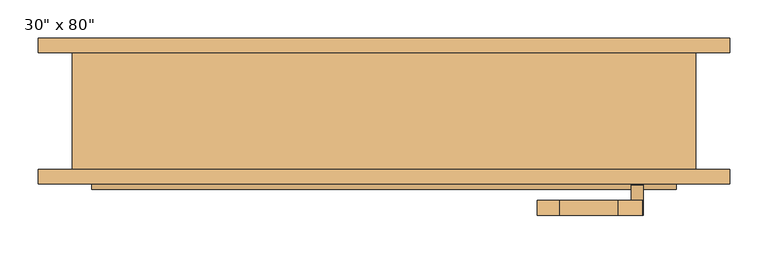
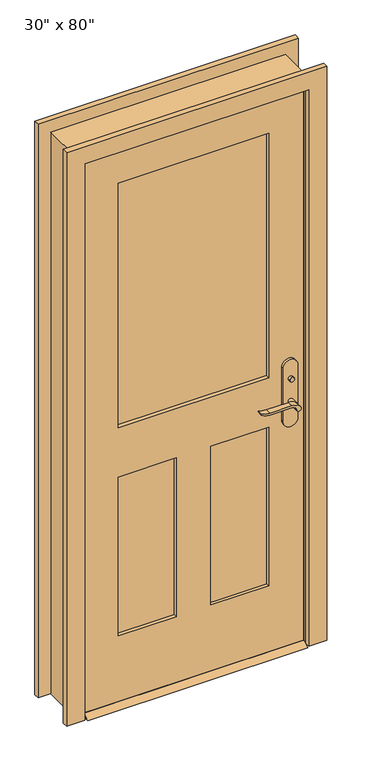
"""IFC4 building model written with IfcOpenShell, lengths in millimetres: door geometry."""

from ifc_helpers import new_model, si_unit, point, frame, frame_2d, origin, place, context, project, spatial, polyline, circle_curve, trimmed, segment, composite_curve, outline, extrude, faceted_brep, source, transform, mapped, element, save


def door_ce1fc124(model_context):
    return source(origin(), model_context, "Body", "SolidModel", [
        extrude(outline(polyline([(-38.1, 12.7), (-12.7, 0.0), (-98.425, 0.0), (-73.025, 12.7), (-38.1, 12.7)])), frame((-381.0, 0.0, 0.0), z_axis=(1.0, 0.0, 0.0), x_axis=(0.0, 1.0, 0.0)), (0.0, 0.0, 1.0), 762.0),
        extrude(outline(polyline([(335.2, -18.1), (335.2, -28.1), (325.2, -28.1), (325.2, -18.1), (335.2, -18.1)])), frame((0.0, 0.0, 981.9), z_axis=(0.0, 0.0, 1.0), x_axis=(1.0, 0.0, 0.0)), (0.0, 0.0, 1.0), 30.0),
        extrude(outline(composite_curve([segment(trimmed(circle_curve(frame_2d((996.9, 330.2)), 8.0), [point((996.9, 322.2))], [point((996.9, 338.2))], False, "CARTESIAN"), True, "CONTINUOUS"), segment(trimmed(circle_curve(frame_2d((996.9, 330.2)), 8.0), [point((996.9, 338.2))], [point((996.9, 322.2))], False, "CARTESIAN"), True, "CONTINUOUS")], self_intersect=False)), frame((0.0, -93.025, 0.0), z_axis=(0.0, 1.0, 0.0), x_axis=(0.0, 0.0, 1.0)), (0.0, 0.0, 1.0), 10.0),
        extrude(outline(composite_curve([segment(trimmed(circle_curve(frame_2d((897.1555521, 306.5324871)), 37.2832219), [point((919.0523287, 336.7081363))], [point((934.4, 304.8325667))], False, "CARTESIAN"), True, "CONTINUOUS"), segment(polyline([(934.4, 304.8325667), (934.4, 228.5564091)]), True, "CONTINUOUS"), segment(trimmed(circle_curve(frame_2d((1017.6850638, 228.6227909)), 83.2850902), [point((934.4, 228.5564091))], [point((939.4, 200.2))], True, "CARTESIAN"), True, "CONTINUOUS"), segment(polyline([(939.4, 200.2), (936.6135558, 200.2)]), True, "CONTINUOUS"), segment(trimmed(circle_curve(frame_2d((986.6709207, 232.1396612)), 59.3791355), [point((936.6135558, 200.2))], [point((927.4, 228.5564091))], False, "CARTESIAN"), True, "CONTINUOUS"), segment(polyline([(927.4, 228.5564091), (927.4, 304.8138099)]), True, "CONTINUOUS"), segment(trimmed(circle_curve(frame_2d((909.2738613, 304.8138099)), 18.1261387), [point((927.4, 304.8138099))], [point((914.4, 322.2))], True, "CARTESIAN"), True, "CONTINUOUS"), segment(trimmed(circle_curve(frame_2d((914.4, 330.2)), 8.0), [point((914.4, 322.2))], [point((919.0523287, 336.7081363))], False, "CARTESIAN"), True, "CONTINUOUS")], self_intersect=False)), frame((0.0, 1.9, 0.0), z_axis=(0.0, 1.0, 0.0), x_axis=(0.0, 0.0, 1.0)), (0.0, 0.0, 1.0), 20.0),
        extrude(outline(composite_curve([segment(trimmed(circle_curve(frame_2d((914.4, 330.2)), 8.0), [point((914.3999903, 322.2))], [point((919.0523287, 336.7081363))], False, "CARTESIAN"), True, "CONTINUOUS"), segment(trimmed(circle_curve(frame_2d((897.1555521, 306.5324871)), 37.2832219), [point((919.0523287, 336.7081363))], [point((934.4, 304.8325667))], False, "CARTESIAN"), True, "CONTINUOUS"), segment(polyline([(934.4, 304.8325667), (934.4, 228.5564091)]), True, "CONTINUOUS"), segment(trimmed(circle_curve(frame_2d((1017.6850638, 228.6227909)), 83.2850902), [point((934.4, 228.5564091))], [point((939.4, 200.2))], True, "CARTESIAN"), True, "CONTINUOUS"), segment(polyline([(939.4, 200.2), (936.6135558, 200.2)]), True, "CONTINUOUS"), segment(trimmed(circle_curve(frame_2d((986.6709207, 232.1396612)), 59.3791355), [point((936.6135558, 200.2))], [point((927.4, 228.5564091))], False, "CARTESIAN"), True, "CONTINUOUS"), segment(polyline([(927.4, 228.5564091), (927.4, 304.8138122)]), True, "CONTINUOUS"), segment(trimmed(circle_curve(frame_2d((909.2738682, 304.8138122)), 18.1261318), [point((927.4, 304.8138122))], [point((914.3999903, 322.2))], True, "CARTESIAN"), True, "CONTINUOUS")], self_intersect=False)), frame((0.0, -133.025, 0.0), z_axis=(0.0, 1.0, 0.0), x_axis=(0.0, 0.0, 1.0)), (0.0, 0.0, 1.0), 20.0),
        extrude(outline(composite_curve([segment(trimmed(circle_curve(frame_2d((914.4, 330.2)), 8.0), [point((914.4, 322.2))], [point((914.4, 338.2))], False, "CARTESIAN"), True, "CONTINUOUS"), segment(trimmed(circle_curve(frame_2d((914.4, 330.2)), 8.0), [point((914.4, 338.2))], [point((914.4, 322.2))], False, "CARTESIAN"), True, "CONTINUOUS")], self_intersect=False)), frame((0.0, -28.1, 0.0), z_axis=(0.0, 1.0, 0.0), x_axis=(0.0, 0.0, 1.0)), (0.0, 0.0, 1.0), 30.0),
        extrude(outline(composite_curve([segment(trimmed(circle_curve(frame_2d((914.4, 330.2)), 8.0), [point((914.4, 322.2))], [point((914.4, 338.2))], False, "CARTESIAN"), True, "CONTINUOUS"), segment(trimmed(circle_curve(frame_2d((914.4, 330.2)), 8.0), [point((914.4, 338.2))], [point((914.4, 322.2))], False, "CARTESIAN"), True, "CONTINUOUS")], self_intersect=False)), frame((0.0, -113.025, 0.0), z_axis=(0.0, 1.0, 0.0), x_axis=(0.0, 0.0, 1.0)), (0.0, 0.0, 1.0), 30.0),
        extrude(outline(composite_curve([segment(polyline([(844.4, 355.2), (1039.4, 355.2)]), True, "CONTINUOUS"), segment(trimmed(circle_curve(frame_2d((1039.4, 330.2)), 25.0), [point((1039.4, 355.2))], [point((1039.4, 305.2))], False, "CARTESIAN"), True, "CONTINUOUS"), segment(polyline([(1039.4, 305.2), (844.4, 305.2)]), True, "CONTINUOUS"), segment(trimmed(circle_curve(frame_2d((844.4, 330.2)), 25.0), [point((844.4, 305.2))], [point((844.4, 355.2))], False, "CARTESIAN"), True, "CONTINUOUS")], self_intersect=False)), frame((0.0, -38.1, 0.0), z_axis=(0.0, 1.0, 0.0), x_axis=(0.0, 0.0, 1.0)), (0.0, 0.0, 1.0), 10.0),
        extrude(outline(composite_curve([segment(polyline([(844.4, 355.2), (1039.4, 355.2)]), True, "CONTINUOUS"), segment(trimmed(circle_curve(frame_2d((1039.4, 330.2)), 25.0), [point((1039.4, 355.2))], [point((1039.4, 305.2))], False, "CARTESIAN"), True, "CONTINUOUS"), segment(polyline([(1039.4, 305.2), (844.4, 305.2)]), True, "CONTINUOUS"), segment(trimmed(circle_curve(frame_2d((844.4, 330.2)), 25.0), [point((844.4, 305.2))], [point((844.4, 355.2))], False, "CARTESIAN"), True, "CONTINUOUS")], self_intersect=False)), frame((0.0, -83.025, 0.0), z_axis=(0.0, 1.0, 0.0), x_axis=(0.0, 0.0, 1.0)), (0.0, 0.0, 1.0), 10.0),
        extrude(outline(polyline([(2032.0, -381.0), (12.7, -381.0), (12.7, 381.0), (2032.0, 381.0), (2032.0, -381.0)]), holes=[polyline([(1016.0, -260.35), (1911.35, -260.35), (1911.35, 260.35), (1016.0, 260.35), (1016.0, -260.35)]), polyline([(835.025, -60.325), (254.0, -60.325), (254.0, -260.35), (835.025, -260.35), (835.025, -60.325)]), polyline([(835.025, 260.35), (254.0, 260.35), (254.0, 60.325), (835.025, 60.325), (835.025, 260.35)])]), frame((0.0, -73.025, 0.0), z_axis=(0.0, 1.0, 0.0), x_axis=(0.0, 0.0, 1.0)), (0.0, 0.0, 1.0), 34.925),
        faceted_brep([(406.4, -73.025, 0.0), (381.0, -73.025, 0.0), (381.0, -38.1, 0.0), (368.3, -38.1, 0.0), (368.3, -3.175, 0.0), (381.0, -3.175, 0.0), (381.0, 79.375, 0.0), (406.4, 79.375, 0.0), (406.4, 79.375, 2057.4), (406.4, -73.025, 2057.4), (381.0, 79.375, 2032.0), (-381.0, 79.375, 2032.0), (-381.0, 79.375, 0.0), (-406.4, 79.375, 0.0), (-406.4, 79.375, 2057.4), (381.0, -3.175, 2032.0), (368.3, -3.175, 2019.3), (-368.3, -3.175, 2019.3), (-368.3, -3.175, 0.0), (-381.0, -3.175, 0.0), (-381.0, -3.175, 2032.0), (368.3, -38.1, 2019.3), (381.0, -38.1, 2032.0), (-381.0, -38.1, 2032.0), (-381.0, -38.1, 0.0), (-368.3, -38.1, 0.0), (-368.3, -38.1, 2019.3), (381.0, -73.025, 2032.0), (-406.4, -73.025, 2057.4), (-406.4, -73.025, 0.0), (-381.0, -73.025, 0.0), (-381.0, -73.025, 2032.0)], [[[0, 1, 2, 3, 4, 5, 6, 7]], [[7, 8, 9, 0]], [[6, 10, 11, 12, 13, 14, 8, 7]], [[5, 15, 10, 6]], [[4, 16, 17, 18, 19, 20, 15, 5]], [[3, 21, 16, 4]], [[2, 22, 23, 24, 25, 26, 21, 3]], [[1, 27, 22, 2]], [[0, 9, 28, 29, 30, 31, 27, 1]], [[8, 14, 28, 9]], [[15, 20, 11, 10]], [[21, 26, 17, 16]], [[27, 31, 23, 22]], [[29, 13, 12, 19, 18, 25, 24, 30]], [[14, 13, 29, 28]], [[20, 19, 12, 11]], [[26, 25, 18, 17]], [[31, 30, 24, 23]]]),
        extrude(outline(polyline([(-60.325, -49.7416667), (-60.325, -61.3833333), (-260.35, -61.3833333), (-260.35, -49.7416667), (-60.325, -49.7416667)])), frame((0.0, 0.0, 254.0), z_axis=(0.0, 0.0, 1.0), x_axis=(1.0, 0.0, 0.0)), (0.0, 0.0, 1.0), 581.025),
        extrude(outline(polyline([(260.35, -49.7416667), (260.35, -61.3833333), (60.325, -61.3833333), (60.325, -49.7416667), (260.35, -49.7416667)])), frame((0.0, 0.0, 254.0), z_axis=(0.0, 0.0, 1.0), x_axis=(1.0, 0.0, 0.0)), (0.0, 0.0, 1.0), 581.025),
        extrude(outline(polyline([(260.35, -52.07), (260.35, -59.055), (-260.35, -59.055), (-260.35, -52.07), (260.35, -52.07)])), frame((0.0, 0.0, 1016.0), z_axis=(0.0, 0.0, 1.0), x_axis=(1.0, 0.0, 0.0)), (0.0, 0.0, 1.0), 895.35),
        extrude(outline(polyline([(0.0, -387.35), (2038.35, -387.35), (2038.35, 387.35), (0.0, 387.35), (0.0, 450.85), (2101.85, 450.85), (2101.85, -450.85), (0.0, -450.85), (0.0, -387.35)])), frame((0.0, 79.375, 0.0), z_axis=(0.0, 1.0, 0.0), x_axis=(0.0, 0.0, 1.0)), (0.0, 0.0, 1.0), 19.05),
        extrude(outline(polyline([(0.0, -387.35), (2038.35, -387.35), (2038.35, 387.35), (0.0, 387.35), (0.0, 450.85), (2101.85, 450.85), (2101.85, -450.85), (0.0, -450.85), (0.0, -387.35)])), frame((0.0, -92.075, 0.0), z_axis=(0.0, 1.0, 0.0), x_axis=(0.0, 0.0, 1.0)), (0.0, 0.0, 1.0), 19.05),
    ])


if __name__ == "__main__":
    model = new_model("IFC4")
    model_context = context("Model", 3, world=origin())
    ifc_project = project(units=[si_unit("LENGTHUNIT", "METRE", prefix="MILLI")], contexts=[model_context])
    site = spatial("IfcSite", under=ifc_project)
    building = spatial("IfcBuilding", under=site)
    placement = place(None, origin())
    door_shape = door_ce1fc124(model_context)
    element("IfcDoor", 1, ObjectType="30\" x 80\"", at=placement, inside=building, context=model_context, shape_type="MappedRepresentation", body=[
        mapped(door_shape, transform((0.0, 0.0, 0.0), x_axis=(1.0, 0.0, 0.0), y_axis=(0.0, 1.0, 0.0), z_axis=(0.0, 0.0, 1.0))),
    ])
    save(model, "model.ifc")

# Revit data of these elements
# Type "30\" x 80\""
#   Type Mark = "8"
#   Assembly Code = "B2030100"
#   Analytic Construction = "French door, wood frame with single glass"
#   Top Rail = 0' - 4 3/4"
#   Threshold Offset [instance default] = 0' - 0 1/2"
#   Thickness = 0' - 1 3/8"
#   Thermal Resistance (R) = 1.0696 (h·ft²·°F)/BTU
#   Swing Angle [instance default] = 90.00°
#   Stiles = 0' - 4 3/4"
#   Rough Width = 2' - 8"
#   Rough Height = 6' - 9"
#   Lock Rail = 0' - 7 1/8"
#   Height = 6' - 8"
#   Width = 2' - 6"
#   Heat Transfer Coefficient (U) = 0.9350 BTU/(h·ft²·°F)
#   Door Offset [instance default] = 0' - 0"
#   Bottom Rail = 0' - 9 1/2"
#   Threshold [instance default] = yes
#   Function = 1
#   Exterior Trim [instance default] = yes
#   Trim Material = Cherry
#   Threshold Material = Cherry
#   Panel Material = Cherry
#   Glazing = Glass
#   Frame Material = Cherry
#   Door Handle Material = Aluminum
#   Visual Light Transmittance = 0
#   Solar Heat Gain Coefficient = 0
#   Wall Closure = (empty or 0)
#   Construction Type = (empty or 0)
# Element 1 (IfcDoor, "30\" x 80\"")
#   Materials on its faces: "Cherry", "Aluminum", "Glass"
# Materials
#   "Cherry": class "Wood", colour RGB 226 177 128, transparency 0, Description = "Prunus Serotina", Cost = 0
#   "Glass": class "Glass", colour RGB 0 128 192, transparency 0.75, Description = "Soda Lime Glass", Cost = 0
#   "Aluminum": class "Metal", colour RGB 247 247 247, transparency 0, Description = "Aluminum 6061", Cost = 0
